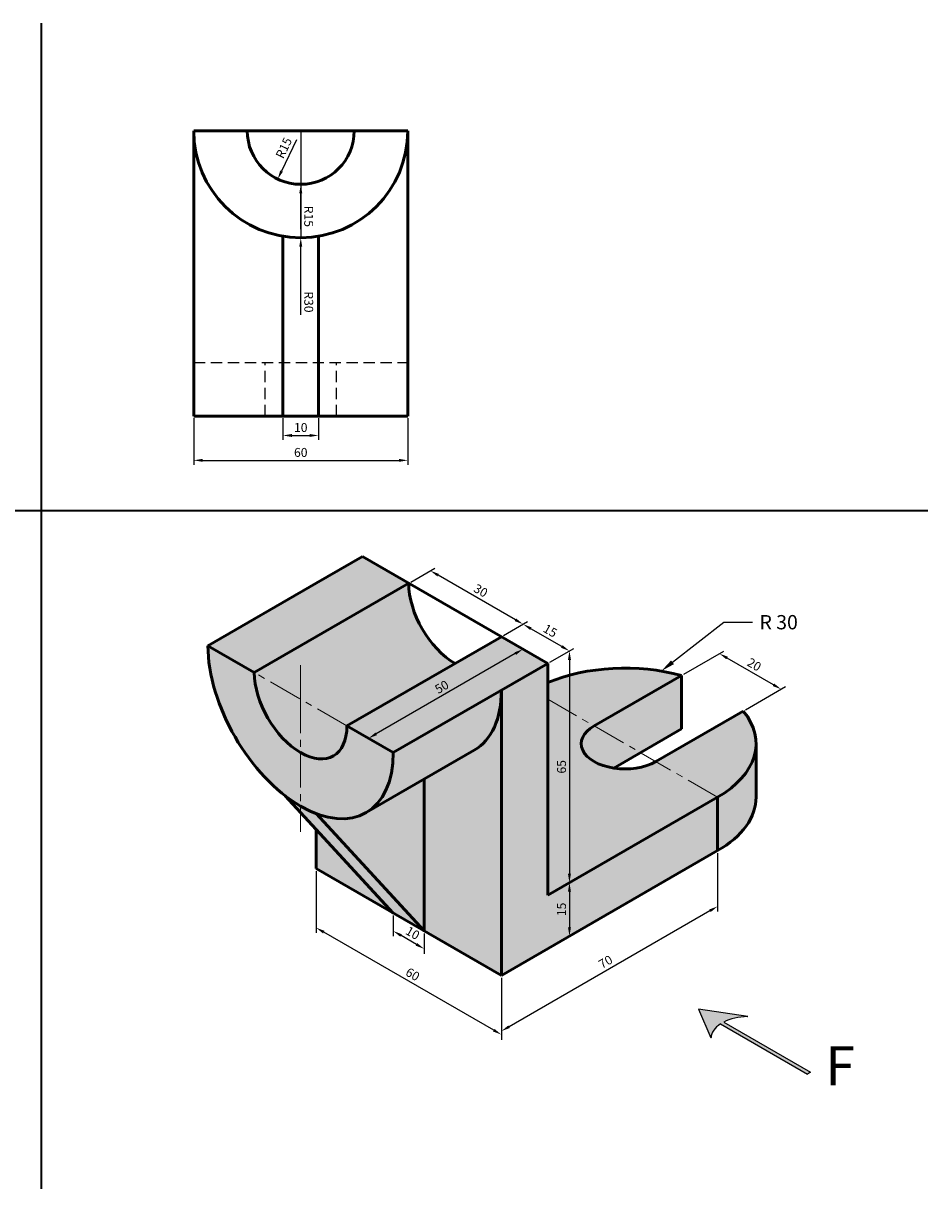
# Model space of a CAD drawing. Units: millimetres. Extents: x 2100 to 2598, y 2059 to 2386.
# Tile 1 of 1: x 2345 to 2598.5, y 2059.2 to 2386.1. Entities that reach past the tile are written whole.
import ezdxf
from ezdxf import colors
from ezdxf.entities.mleader import LeaderData, LeaderLine
from ezdxf.math import Vec2, Vec3

# ---------------------------------------------------------------- set-up
doc = ezdxf.new("R2010")
doc.units = ezdxf.units.MM
doc.linetypes.add('CENTER', pattern=[50.800000000000004, 31.75, -6.349999999999999, 6.349999999999999, -6.349999999999999])
doc.linetypes.add('HIDDEN', pattern=[9.524999999999999, 6.349999999999999, -3.174999999999999])
for name, color, linetype, lineweight in [('M-CNTR', 1, 'CENTER', 18), ('M-DIMS', 2, 'Continuous', 25), ('M-HATC', 8, 'Continuous', 18), ('M-HIDN', 4, 'HIDDEN', 25), ('M-OUTL', 7, 'Continuous', 50), ('M-SYMB', 3, 'Continuous', 25), ('M-TEXT', 3, 'Continuous', 25), ('M-TTLB', 7, 'Continuous', 35)]:
    doc.layers.add(name, color=color, linetype=linetype, lineweight=lineweight)
doc.styles.get("Standard").update_dxf_attribs({"font": 'arial.ttf'})
doc.dimstyles.new('ISO-25', dxfattribs={"dimtxt": 2.5, "dimasz": 2.5, "dimexe": 1.25, "dimexo": 0.625, "dimtad": 1, "dimtxsty": 'Standard', "dimcen": 2.5, "dimadec": 0, "dimazin": 0, "dimtfac": 1, "dimtmove": 0, "dimatfit": 3, "dimfxl": 1, "dimarcsym": 0})

# ---------------------------------------------------------------- blocks, each defined once
blk = doc.blocks.new('*D1')
at = {"layer": 'Defpoints', "color": 0, "transparency": 16777216}
for p in [(2539.605304126091, 2154.015574950749), (2478.98352586118, 2119.015574950749), (2478.98352586118, 2103.385647397557)]:
    blk.add_point(p, dxfattribs=at)
at = {"layer": 'M-DIMS', "color": 0, "lineweight": -2, "transparency": 16777216}
for p, q in [((2539.605304126091, 2153.293887114262), (2539.605304126091, 2136.942271724583)), ((2537.44024061663, 2137.135647397557), (2481.148589370641, 2104.635647397557)), ((2478.98352586118, 2118.293887114262), (2478.98352586118, 2101.942271724583))]:
    blk.add_line(p, q, dxfattribs=at)
at = {"layer": 'M-DIMS', "color": 0, "transparency": 16777216}
for points in [[(2537.231907283296, 2137.4964913158), (2537.648573949963, 2136.774803479313), (2539.605304126091, 2138.385647397557)], [(2480.940256037307, 2104.9964913158), (2481.356922703974, 2104.274803479313), (2478.98352586118, 2103.385647397557)]]:
    blk.add_solid(points, dxfattribs=at)
at = {"layer": 'M-DIMS', "color": 0, "transparency": 16777216, "insert": (2508.343698758983, 2122.532336219554), "char_height": 2.5, "attachment_point": 5, "rotation": 30.000000000000068}
blk.add_mtext('70', dxfattribs=at)
blk = doc.blocks.new('*D2')
at = {"layer": 'Defpoints', "color": 0, "transparency": 16777216}
for p in [(2427.022001634114, 2149.01557495075), (2427.022001634114, 2132.403009386933), (2478.98352586118, 2119.015574950749)]:
    blk.add_point(p, dxfattribs=at)
at = {"layer": 'M-DIMS', "color": 0, "lineweight": -2, "transparency": 16777216}
for p, q in [((2427.022001634114, 2148.293887114263), (2427.022001634114, 2130.959633713958)), ((2476.818462351719, 2103.653009386933), (2429.187065143575, 2131.153009386932)), ((2478.98352586118, 2118.293887114262), (2478.98352586118, 2100.959633713959))]:
    blk.add_line(p, q, dxfattribs=at)
at = {"layer": 'M-DIMS', "color": 0, "transparency": 16777216}
for points in [[(2429.395398476908, 2131.513853305176), (2428.978731810242, 2130.79216546869), (2427.022001634114, 2132.403009386933)], [(2477.026795685052, 2104.013853305176), (2476.610129018386, 2103.29216546869), (2478.98352586118, 2102.403009386933)]]:
    blk.add_solid(points, dxfattribs=at)
at = {"layer": 'M-DIMS', "color": 0, "transparency": 16777216, "insert": (2453.953479982299, 2119.049698208931), "char_height": 2.5, "attachment_point": 5, "rotation": 330.0000000000001}
blk.add_mtext('60', dxfattribs=at)
blk = doc.blocks.new('*D3')
at = {"layer": 'Defpoints', "color": 0, "transparency": 16777216}
for p in [(2448.672636728725, 2136.515574950749), (2448.672636728725, 2131.469743862794), (2457.332890766569, 2131.515574950749)]:
    blk.add_point(p, dxfattribs=at)
at = {"layer": 'M-DIMS', "color": 0, "lineweight": -2, "transparency": 16777216}
for p, q in [((2448.672636728725, 2135.793887114262), (2448.672636728725, 2130.026368189821)), ((2455.167827257108, 2127.719743862795), (2450.837700238186, 2130.219743862795)), ((2457.332890766569, 2130.793887114263), (2457.332890766569, 2125.026368189821))]:
    blk.add_line(p, q, dxfattribs=at)
at = {"layer": 'M-DIMS', "color": 0, "transparency": 16777216}
for points in [[(2451.046033571519, 2130.580587781038), (2450.629366904853, 2129.858899944551), (2448.672636728725, 2131.469743862794)], [(2455.376160590442, 2128.080587781038), (2454.959493923775, 2127.358899944551), (2457.332890766569, 2126.469743862795)]]:
    blk.add_solid(points, dxfattribs=at)
at = {"layer": 'M-DIMS', "color": 0, "transparency": 16777216, "insert": (2453.953479982299, 2130.616432684793), "char_height": 2.5, "attachment_point": 5, "rotation": 330.0000000000001}
blk.add_mtext('10', dxfattribs=at)
blk = doc.blocks.new('*D4')
at = {"layer": 'Defpoints', "color": 0, "transparency": 16777216}
for p in [(2491.973906917947, 2206.515574950749), (2441.723938290984, 2185.527407864297), (2448.672636728725, 2181.515574950749)]:
    blk.add_point(p, dxfattribs=at)
at = {"layer": 'M-DIMS', "color": 0, "lineweight": -2, "transparency": 16777216}
for p, q in [((2491.348906917947, 2206.876418868993), (2483.775208480207, 2211.249095700784)), ((2482.860144970745, 2209.277407864297), (2443.889001800445, 2186.777407864297)), ((2448.047636728726, 2181.876418868993), (2440.473938290984, 2186.249095700784))]:
    blk.add_line(p, q, dxfattribs=at)
at = {"layer": 'M-DIMS', "color": 0, "transparency": 16777216}
for points in [[(2482.651811637412, 2209.638251782541), (2483.068478304079, 2208.916563946054), (2485.025208480207, 2210.527407864297)], [(2443.680668467112, 2187.138251782541), (2444.097335133779, 2186.416563946053), (2441.723938290984, 2185.527407864297)]]:
    blk.add_solid(points, dxfattribs=at)
at = {"layer": 'M-DIMS', "color": 0, "transparency": 16777216, "insert": (2462.423857150943, 2199.674096686295), "char_height": 2.5, "attachment_point": 5, "rotation": 29.999999999999872}
blk.add_mtext('50', dxfattribs=at)
blk = doc.blocks.new('*D5')
at = {"layer": 'Defpoints', "color": 0, "transparency": 16777216}
for p in [(2485.074026823124, 2217.531927320627), (2478.98352586118, 2214.015574950749), (2491.973906917947, 2206.515574950749)]:
    blk.add_point(p, dxfattribs=at)
at = {"layer": 'M-DIMS', "color": 0, "lineweight": -2, "transparency": 16777216}
for p, q in [((2479.608525861181, 2214.376418868993), (2486.324026823124, 2218.253615157115)), ((2495.89934437043, 2211.281927320627), (2487.239090332585, 2216.281927320627)), ((2492.598906917947, 2206.876418868993), (2499.314407879891, 2210.753615157114))]:
    blk.add_line(p, q, dxfattribs=at)
at = {"layer": 'M-DIMS', "color": 0, "transparency": 16777216}
for points in [[(2487.447423665918, 2216.642771238871), (2487.030756999252, 2215.921083402384), (2485.074026823124, 2217.531927320627)], [(2496.107677703763, 2211.642771238871), (2495.691011037096, 2210.921083402384), (2498.064407879891, 2210.031927320627)]]:
    blk.add_solid(points, dxfattribs=at)
at = {"layer": 'M-DIMS', "color": 0, "transparency": 16777216, "insert": (2492.519933586159, 2215.428616142625), "char_height": 2.5, "attachment_point": 5, "rotation": 330.0000000000001}
blk.add_mtext('15', dxfattribs=at)
blk = doc.blocks.new('*D6')
at = {"layer": 'Defpoints', "color": 0, "transparency": 16777216}
for p in [(2491.973906917948, 2206.515574950751), (2498.064407879893, 2145.031927320629), (2491.973906917948, 2141.51557495075)]:
    blk.add_point(p, dxfattribs=at)
at = {"layer": 'M-DIMS', "color": 0, "lineweight": -2, "transparency": 16777216}
for p, q in [((2492.598906917948, 2206.876418868994), (2499.314407879893, 2210.753615157116)), ((2498.064407879893, 2207.531927320629), (2498.064407879893, 2147.531927320629)), ((2492.598906917948, 2141.876418868994), (2499.314407879893, 2145.753615157116))]:
    blk.add_line(p, q, dxfattribs=at)
at = {"layer": 'M-DIMS', "color": 0, "transparency": 16777216}
for points in [[(2497.647741213226, 2207.531927320629), (2498.481074546559, 2207.531927320629), (2498.064407879893, 2210.031927320629)], [(2497.647741213226, 2147.531927320629), (2498.481074546559, 2147.531927320629), (2498.064407879893, 2145.031927320629)]]:
    blk.add_solid(points, dxfattribs=at)
at = {"layer": 'M-DIMS', "color": 0, "transparency": 16777216, "insert": (2496.162975410588, 2177.531927320628), "char_height": 2.5, "attachment_point": 5, "rotation": 90}
blk.add_mtext('65', dxfattribs=at)
blk = doc.blocks.new('*D7')
at = {"layer": 'Defpoints', "color": 0, "transparency": 16777216}
for p in [(2459.093264709591, 2232.531927320627), (2453.002763747647, 2229.01557495075), (2478.98352586118, 2214.015574950749)]:
    blk.add_point(p, dxfattribs=at)
at = {"layer": 'M-DIMS', "color": 0, "lineweight": -2, "transparency": 16777216}
for p, q in [((2453.627763747647, 2229.376418868993), (2460.343264709591, 2233.253615157114)), ((2482.908963313662, 2218.781927320627), (2461.258328219052, 2231.281927320627)), ((2479.608525861181, 2214.376418868993), (2486.324026823123, 2218.253615157115))]:
    blk.add_line(p, q, dxfattribs=at)
at = {"layer": 'M-DIMS', "color": 0, "transparency": 16777216}
for points in [[(2461.466661552385, 2231.642771238871), (2461.049994885719, 2230.921083402384), (2459.093264709591, 2232.531927320627)], [(2483.117296646996, 2219.142771238871), (2482.70062998033, 2218.421083402384), (2485.074026823124, 2217.531927320627)]]:
    blk.add_solid(points, dxfattribs=at)
at = {"layer": 'M-DIMS', "color": 0, "transparency": 16777216, "insert": (2473.03478833116, 2226.679354568106), "char_height": 2.5, "attachment_point": 5, "rotation": 330.0000000000001}
blk.add_mtext('30', dxfattribs=at)
blk = doc.blocks.new('*D8')
at = {"layer": 'Defpoints', "color": 0, "transparency": 16777216}
for p in [(2540.093305136287, 2209.297322465351), (2529.459185402545, 2203.157710574481), (2546.779693478234, 2193.15771057448)]:
    blk.add_point(p, dxfattribs=at)
at = {"layer": 'M-DIMS', "color": 0, "lineweight": -2, "transparency": 16777216}
for p, q in [((2530.084185402545, 2203.518554492724), (2541.343305136287, 2210.019010301838)), ((2555.248749702514, 2200.547322465352), (2542.258368645748, 2208.047322465351)), ((2547.404693478234, 2193.518554492724), (2558.663813211976, 2200.019010301839))]:
    blk.add_line(p, q, dxfattribs=at)
at = {"layer": 'M-DIMS', "color": 0, "transparency": 16777216}
for points in [[(2542.466701979082, 2208.408166383595), (2542.050035312414, 2207.686478547108), (2540.093305136287, 2209.297322465351)], [(2555.457083035848, 2200.908166383595), (2555.040416369181, 2200.186478547108), (2557.413813211976, 2199.297322465351)]]:
    blk.add_solid(points, dxfattribs=at)
at = {"layer": 'M-DIMS', "color": 0, "transparency": 16777216, "insert": (2549.704275408783, 2205.94401128735), "char_height": 2.5, "attachment_point": 5, "rotation": 330.0000000000001}
blk.add_mtext('20', dxfattribs=at)
blk = doc.blocks.new('*D9')
at = {"layer": 'Defpoints', "color": 0, "transparency": 16777216}
for p in [(2491.973906917948, 2141.51557495075), (2498.064407879894, 2130.031927320629), (2491.973906917948, 2126.515574950751)]:
    blk.add_point(p, dxfattribs=at)
at = {"layer": 'M-DIMS', "color": 0, "lineweight": -2, "transparency": 16777216}
for p, q in [((2492.598906917948, 2141.876418868994), (2499.314407879894, 2145.753615157116)), ((2498.064407879894, 2142.531927320629), (2498.064407879894, 2132.53192732063)), ((2492.598906917948, 2126.876418868994), (2499.314407879894, 2130.753615157117))]:
    blk.add_line(p, q, dxfattribs=at)
at = {"layer": 'M-DIMS', "color": 0, "transparency": 16777216}
for points in [[(2497.647741213227, 2142.531927320629), (2498.48107454656, 2142.531927320629), (2498.064407879894, 2145.031927320629)], [(2497.647741213227, 2132.53192732063), (2498.48107454656, 2132.53192732063), (2498.064407879894, 2130.031927320629)]]:
    blk.add_solid(points, dxfattribs=at)
at = {"layer": 'M-DIMS', "color": 0, "transparency": 16777216, "insert": (2496.16297541059, 2137.531927320629), "char_height": 2.5, "attachment_point": 5, "rotation": 90}
blk.add_mtext('15', dxfattribs=at)
blk = doc.blocks.new('*D15')
at = {"layer": 'Defpoints', "color": 0, "transparency": 16777216}
for p in [(2417.737806239899, 2275.948119333525), (2427.737806239898, 2275.948119333525), (2427.737806239898, 2270.485342262566)]:
    blk.add_point(p, dxfattribs=at)
at = {"layer": 'M-DIMS', "color": 0, "lineweight": -2, "transparency": 16777216}
for p, q in [((2417.737806239899, 2275.323119333525), (2417.737806239899, 2269.235342262566)), ((2427.737806239898, 2275.323119333525), (2427.737806239898, 2269.235342262566)), ((2420.237806239899, 2270.485342262566), (2425.237806239899, 2270.485342262566))]:
    blk.add_line(p, q, dxfattribs=at)
at = {"layer": 'M-DIMS', "color": 0, "transparency": 16777216}
for points in [[(2420.237806239899, 2270.902008929232), (2420.237806239899, 2270.068675595899), (2417.737806239899, 2270.485342262566)], [(2425.237806239899, 2270.902008929232), (2425.237806239899, 2270.068675595899), (2427.737806239898, 2270.485342262566)]]:
    blk.add_solid(points, dxfattribs=at)
at = {"layer": 'M-DIMS', "color": 0, "transparency": 16777216, "insert": (2422.737806239898, 2272.38677473187), "char_height": 2.5, "attachment_point": 5}
blk.add_mtext('10', dxfattribs=at)
blk = doc.blocks.new('*D16')
at = {"layer": 'Defpoints', "color": 0, "transparency": 16777216}
for p in [(2392.737806239899, 2275.948119333525), (2452.737806239899, 2275.948119333525), (2452.737806239899, 2263.507971917901)]:
    blk.add_point(p, dxfattribs=at)
at = {"layer": 'M-DIMS', "color": 0, "lineweight": -2, "transparency": 16777216}
for p, q in [((2392.737806239899, 2275.323119333525), (2392.737806239899, 2262.257971917901)), ((2452.737806239899, 2275.323119333525), (2452.737806239899, 2262.257971917901)), ((2395.237806239899, 2263.507971917901), (2450.237806239899, 2263.507971917901))]:
    blk.add_line(p, q, dxfattribs=at)
at = {"layer": 'M-DIMS', "color": 0, "transparency": 16777216}
for points in [[(2395.237806239899, 2263.924638584568), (2395.237806239899, 2263.091305251235), (2392.737806239899, 2263.507971917901)], [(2450.237806239899, 2263.924638584568), (2450.237806239899, 2263.091305251235), (2452.737806239899, 2263.507971917901)]]:
    blk.add_solid(points, dxfattribs=at)
at = {"layer": 'M-DIMS', "color": 0, "transparency": 16777216, "insert": (2422.737806239898, 2265.409404387206), "char_height": 2.5, "attachment_point": 5}
blk.add_mtext('60', dxfattribs=at)
blk = doc.blocks.new('*D17')
at = {"layer": 'Defpoints', "color": 0, "transparency": 16777216}
for p in [(2422.737806239896, 2355.948119333517), (2416.274107555597, 2342.412218945352)]:
    blk.add_point(p, dxfattribs=at)
at = {"layer": 'M-DIMS', "color": 0, "lineweight": -2, "transparency": 16777216}
blk.add_line((2421.549561495412, 2353.459766567759), (2417.351390669647, 2344.668202343381), dxfattribs=at)
at = {"layer": 'M-DIMS', "color": 0, "transparency": 16777216}
blk.add_solid([(2416.975393436643, 2344.847749529055), (2417.727387902653, 2344.488655157705), (2416.274107555597, 2342.412218945352)], dxfattribs=at)
at = {"layer": 'M-DIMS', "color": 0, "transparency": 16777216, "insert": (2418.273277606266, 2351.01132859126), "char_height": 2.5, "attachment_point": 5, "rotation": 64.47446902836414}
blk.add_mtext('R15', dxfattribs=at)
blk = doc.blocks.new('*D22')
at = {"layer": 'Defpoints', "color": 0, "transparency": 16777216}
for p in [(2422.737806000001, 2355.948119000002), (2422.738000000001, 2340.948119000001)]:
    blk.add_point(p, dxfattribs=at)
at = {"layer": 'M-DIMS', "color": 0, "lineweight": -2, "transparency": 16777216}
for p, q in [((2422.737806000001, 2355.948119000002), (2422.738000000001, 2340.948119000001)), ((2422.738163234812, 2328.326870706377), (2422.738032333334, 2338.44811900021))]:
    blk.add_line(p, q, dxfattribs=at)
at = {"layer": 'M-DIMS', "color": 0, "transparency": 16777216}
blk.add_solid([(2423.154698999966, 2338.448124389099), (2422.321365666702, 2338.448113611321), (2422.738000000001, 2340.948119000001)], dxfattribs=at)
at = {"layer": 'M-DIMS', "color": 0, "transparency": 16777216, "insert": (2424.639548869146, 2331.948143592613), "char_height": 2.5, "attachment_point": 5, "rotation": 270.00074102541396}
blk.add_mtext('R15', dxfattribs=at)
blk = doc.blocks.new('*D23')
at = {"layer": 'Defpoints', "color": 0, "transparency": 16777216}
for p in [(2422.737806000003, 2355.948119000001), (2422.738000000002, 2325.948119000003)]:
    blk.add_point(p, dxfattribs=at)
at = {"layer": 'M-DIMS', "color": 0, "lineweight": -2, "transparency": 16777216}
for p, q in [((2422.737806000003, 2355.948119000001), (2422.738000000002, 2325.948119000003)), ((2422.738139729186, 2304.340513270576), (2422.73801616667, 2323.448119000055))]:
    blk.add_line(p, q, dxfattribs=at)
at = {"layer": 'M-DIMS', "color": 0, "transparency": 16777216}
blk.add_solid([(2423.154682833327, 2323.448121694499), (2422.321349500011, 2323.44811630561), (2422.738000000002, 2325.948119000003)], dxfattribs=at)
at = {"layer": 'M-DIMS', "color": 0, "transparency": 16777216, "insert": (2424.640401529567, 2307.948131301821), "char_height": 2.5, "attachment_point": 5, "rotation": 270.00037051270704}
blk.add_mtext('R30', dxfattribs=at)

msp = doc.modelspace()

# ---------------------------------------------------------------- hatches: boundary and pattern name
at = {"layer": 'M-HATC'}
h = msp.add_hatch(color=256, dxfattribs=at)
h.dxf.hatch_style = 1
edge = h.paths.add_edge_path()
edge.add_ellipse((2453.002763747647, 2214.015574950749), major_axis=(18.37117307087393, -31.81980515339472), ratio=0.5773502691896212, start_angle=360, end_angle=390)
edge.add_line((2478.98352586118, 2199.015574950749), (2448.672636728725, 2181.515574950749))
edge.add_ellipse((2422.691874615191, 2196.515574950749), major_axis=(18.37117307087387, -31.81980515339462), ratio=0.5773502691896232, start_angle=359.9999999999999, end_angle=390, ccw=False)
edge.add_line((2441.063047686065, 2164.695769797355), (2471.373936818521, 2182.195769797355))
h.paths.add_polyline_path([(2478.98352586118, 2199.015574950749), (2491.973906917948, 2206.515574950749), (2478.98352586118, 2214.01557495075), (2435.682255671958, 2189.01557495075), (2448.672636728725, 2181.515574950749)])
edge = h.paths.add_edge_path()
edge.add_ellipse((2453.002763747647, 2214.015574950749), major_axis=(18.37117307087393, -31.81980515339472), ratio=0.5773502691896212, start_angle=360, end_angle=390, ccw=False)
edge.add_line((2471.373936818521, 2182.195769797355), (2457.332890766569, 2174.089168079557))
edge.add_line((2457.332890766569, 2174.089168079557), (2457.332890766569, 2131.515574950749))
edge.add_line((2457.332890766569, 2131.515574950749), (2478.98352586118, 2119.015574950749))
edge.add_line((2478.98352586118, 2119.015574950749), (2478.98352586118, 2199.015574950749))
h.paths.add_polyline_path([(2491.973906917947, 2206.515574950749), (2478.98352586118, 2199.015574950749), (2478.98352586118, 2119.015574950749), (2539.605304126091, 2154.015574950749), (2539.605304126091, 2169.01557495075), (2491.973906917947, 2141.51557495075)])
h.paths.add_polyline_path([(2539.605304126091, 2169.01557495075), (2491.973906917947, 2196.51557495075), (2491.973906917947, 2141.51557495075)], flags=17)
edge = h.paths.add_edge_path()
edge.add_ellipse((2513.624542012558, 2184.01557495075), major_axis=(-36.74234614174767, 0), ratio=0.5773502691896243, start_angle=510, end_angle=540)
edge.add_ellipse((2513.624542012558, 2184.01557495075), major_axis=(-36.74234614174767, 0), ratio=0.5773502691896243, start_angle=540, end_angle=195.4155559431911)
edge.add_line((2546.779693478235, 2193.157710574481), (2522.284796050402, 2179.015574950749))
edge.add_line((2522.284796050402, 2179.015574950749), (2539.605304126091, 2169.01557495075))
edge = h.paths.add_edge_path(flags=17)
edge.add_ellipse((2513.624542012558, 2184.01557495075), major_axis=(-36.74234614174767, 0), ratio=0.5773502691896243, start_angle=230.4019697012312, end_angle=321.6340594852775)
edge.add_line((2491.973906917947, 2201.154711451752), (2491.973906917947, 2196.51557495075))
edge.add_line((2491.973906917947, 2196.51557495075), (2504.964287974714, 2189.01557495075))
edge.add_line((2504.964287974714, 2189.01557495075), (2529.459185402545, 2203.15771057448))
edge = h.paths.add_edge_path(flags=16)
edge.add_line((2517.95466903148, 2181.515574950749), (2504.964287974714, 2189.01557495075))
edge.add_ellipse((2513.624542012558, 2184.01557495075), major_axis=(-12.24744871391589, 0), ratio=0.5773502691896119, start_angle=329.9999999999987, end_angle=425.1039093610203)
edge.add_line((2510.45466903148, 2177.185447931827), (2517.95466903148, 2181.515574950749))
edge = h.paths.add_edge_path(flags=16)
edge.add_ellipse((2513.624542012558, 2184.01557495075), major_axis=(-12.24744871391589, 0), ratio=0.5773502691896119, start_angle=425.1039093610203, end_angle=510.0000000000001)
edge.add_line((2522.284796050402, 2179.015574950749), (2517.95466903148, 2181.515574950749))
edge.add_line((2517.95466903148, 2181.515574950749), (2510.45466903148, 2177.185447931827))
edge = h.paths.add_edge_path()
edge.add_line((2550.366888154305, 2169.01557495075), (2550.366888154305, 2184.01557495075))
edge.add_ellipse((2513.624542012558, 2184.01557495075), major_axis=(-36.74234614174767, 0), ratio=0.5773502691896243, start_angle=510.0000000000001, end_angle=540, ccw=False)
edge.add_line((2539.605304126091, 2169.01557495075), (2539.605304126091, 2154.015574950749))
edge.add_ellipse((2513.624542012558, 2169.01557495075), major_axis=(-36.74234614174767, 0), ratio=0.5773502691896243, start_angle=510, end_angle=540)
h.paths.add_polyline_path([(2478.98352586118, 2119.015574950749), (2478.98352586118, 2199.015574950749), (2448.672636728725, 2181.515574950749), (2435.682255671958, 2189.01557495075), (2422.691874615191, 2196.515574950749), (2422.691874615191, 2164.732375880323), (2448.672636728725, 2136.515574950749)], flags=17)
edge = h.paths.add_edge_path()
edge.add_ellipse((2422.691874615191, 2196.515574950749), major_axis=(9.185586535436936, -15.90990257669731), ratio=0.5773502691896232, start_angle=210.0000000000001, end_angle=329.99999999999994, ccw=False)
edge.add_line((2409.701493558425, 2204.01557495075), (2396.711112501658, 2211.51557495075))
edge.add_ellipse((2422.691874615191, 2196.515574950749), major_axis=(18.37117307087387, -31.81980515339462), ratio=0.5773502691896232, start_angle=210, end_angle=320.9153690765151)
edge.add_ellipse((2422.691874615191, 2196.515574950749), major_axis=(18.37117307087387, -31.81980515339462), ratio=0.5773502691896232, start_angle=320.9153690765151, end_angle=329.9999999999999)
edge.add_line((2422.691874615191, 2166.51557495075), (2422.691874615191, 2181.515574950749))
h.paths.add_polyline_path([(2453.002763747647, 2229.01557495075), (2440.012382690881, 2236.515574950749), (2427.022001634114, 2229.01557495075), (2396.711112501658, 2211.51557495075), (2409.701493558425, 2204.01557495075)])
edge = h.paths.add_edge_path()
edge.add_ellipse((2422.691874615191, 2196.515574950749), major_axis=(9.185586535436936, -15.90990257669731), ratio=0.5773502691896232, start_angle=329.9999999999999, end_angle=390)
edge.add_line((2435.682255671958, 2189.01557495075), (2422.691874615191, 2196.515574950749))
edge.add_line((2422.691874615191, 2196.515574950749), (2422.691874615191, 2181.515574950749))
h.paths.add_polyline_path([(2478.98352586118, 2199.015574950749), (2448.672636728725, 2181.515574950749), (2435.682255671958, 2189.01557495075), (2422.691874615191, 2196.515574950749), (2422.691874615191, 2181.515574950749), (2422.691874615191, 2166.51557495075), (2422.691874615191, 2164.732375880323), (2448.672636728725, 2136.515574950749), (2478.98352586118, 2119.015574950749)], flags=17)
h.paths.add_polyline_path([(2427.022001634114, 2160.029575725394), (2427.022001634114, 2149.01557495075), (2448.672636728725, 2136.515574950749)], flags=0)
h = msp.add_hatch(color=256, dxfattribs=at)
h.dxf.hatch_style = 1
edge = h.paths.add_edge_path()
edge.add_ellipse((2465.993144804414, 2221.51557495075), major_axis=(9.185586535436936, -15.90990257669731), ratio=0.5773502691896232, start_angle=210.0000000000001, end_angle=329.99999999999994, ccw=False)
edge.add_line((2453.002763747647, 2229.01557495075), (2409.701493558425, 2204.01557495075))
edge.add_line((2409.701493558425, 2204.01557495075), (2435.682255671958, 2189.01557495075))
edge.add_line((2435.682255671958, 2189.01557495075), (2465.993144804413, 2206.515574950749))
edge = h.paths.add_edge_path()
edge.add_line((2422.691874615191, 2196.515574950749), (2409.701493558425, 2204.01557495075))
edge.add_ellipse((2422.691874615191, 2196.515574950749), major_axis=(9.185586535436936, -15.90990257669731), ratio=0.5773502691896232, start_angle=210, end_angle=329.9999999999999)
edge.add_line((2422.691874615191, 2181.515574950749), (2422.691874615191, 2196.515574950749))
edge = h.paths.add_edge_path()
edge.add_ellipse((2422.691874615191, 2196.515574950749), major_axis=(9.185586535436936, -15.90990257669731), ratio=0.5773502691896232, start_angle=329.9999999999999, end_angle=390)
edge.add_line((2435.682255671958, 2189.01557495075), (2422.691874615191, 2196.515574950749))
edge.add_line((2422.691874615191, 2196.515574950749), (2422.691874615191, 2181.515574950749))
h.paths.add_polyline_path([(2529.459185402545, 2203.157710574481), (2504.964287974714, 2189.01557495075), (2517.95466903148, 2181.515574950749), (2529.459185402545, 2188.157710574481)])
edge = h.paths.add_edge_path()
edge.add_ellipse((2513.624542012558, 2184.01557495075), major_axis=(-12.24744871391589, 0), ratio=0.5773502691896119, start_angle=329.9999999999987, end_angle=425.1039093610203)
edge.add_line((2510.45466903148, 2177.185447931827), (2517.95466903148, 2181.515574950749))
edge.add_line((2517.95466903148, 2181.515574950749), (2504.964287974714, 2189.01557495075))
edge = h.paths.add_edge_path()
edge.add_line((2457.332890766569, 2174.089168079557), (2441.063047686065, 2164.695769797355))
edge.add_ellipse((2422.691874615191, 2196.515574950749), major_axis=(18.37117307087387, -31.81980515339462), ratio=0.5773502691896232, start_angle=337.68717287009406, end_angle=359.9999999999999, ccw=False)
edge.add_line((2427.022001634114, 2164.435176035252), (2457.332890766569, 2131.515574950749))
edge.add_line((2457.332890766569, 2131.515574950749), (2457.332890766569, 2174.089168079557))
edge = h.paths.add_edge_path()
edge.add_ellipse((2422.691874615191, 2196.515574950749), major_axis=(18.37117307087387, -31.81980515339462), ratio=0.5773502691896232, start_angle=329.99999999999994, end_angle=337.68717287009406, ccw=False)
edge.add_line((2422.691874615191, 2166.51557495075), (2422.691874615191, 2164.732375880323))
edge.add_line((2422.691874615191, 2164.732375880323), (2448.672636728725, 2136.515574950749))
edge.add_line((2448.672636728725, 2136.515574950749), (2457.332890766569, 2131.515574950749))
edge.add_line((2457.332890766569, 2131.515574950749), (2427.022001634114, 2164.435176035252))
edge = h.paths.add_edge_path()
edge.add_ellipse((2422.691874615191, 2196.515574950749), major_axis=(18.37117307087387, -31.81980515339462), ratio=0.5773502691896232, start_angle=320.9153690765151, end_angle=329.99999999999994, ccw=False)
edge.add_line((2418.361747596269, 2169.435176035252), (2422.691874615191, 2164.732375880323))
edge.add_line((2422.691874615191, 2164.732375880323), (2422.691874615191, 2166.51557495075))
h = msp.add_hatch(color=256, dxfattribs=at)
h.dxf.hatch_style = 1
edge = h.paths.add_edge_path()
edge.add_ellipse((2422.691874615191, 2196.515574950749), major_axis=(18.37117307087387, -31.81980515339462), ratio=0.5773502691896232, start_angle=359.9999999999999, end_angle=390)
edge.add_line((2448.672636728725, 2181.515574950749), (2435.682255671958, 2189.01557495075))
edge.add_ellipse((2422.691874615191, 2196.515574950749), major_axis=(9.185586535436936, -15.90990257669731), ratio=0.5773502691896232, start_angle=329.99999999999994, end_angle=390, ccw=False)
edge.add_line((2422.691874615191, 2181.515574950749), (2422.691874615191, 2166.51557495075))
edge.add_ellipse((2422.691874615191, 2196.515574950749), major_axis=(18.37117307087387, -31.81980515339462), ratio=0.5773502691896232, start_angle=329.9999999999999, end_angle=337.6871728700941)
edge.add_ellipse((2422.691874615191, 2196.515574950749), major_axis=(18.37117307087387, -31.81980515339462), ratio=0.5773502691896232, start_angle=337.6871728700941, end_angle=359.9999999999999)
h.paths.add_polyline_path([(2427.022001634114, 2160.029575725394), (2427.022001634114, 2149.01557495075), (2448.672636728725, 2136.515574950749)])
at = {"layer": 'M-SYMB'}
h = msp.add_hatch(color=256, dxfattribs=at)
h.dxf.hatch_style = 1
edge = h.paths.add_edge_path()
edge.add_ellipse((2548.340327794889, 2101.348676846816), major_axis=(-10.59557621008401, 0), ratio=0.5773502691896403, start_angle=273.4886162533513, end_angle=327.04442488872957, ccw=False)
edge.add_line((2547.967624843714, 2107.46224993555), (2548.055619139272, 2107.513053465777))
edge.add_line((2548.055619139272, 2107.513053465777), (2534.199212678721, 2109.513053465777))
edge.add_line((2534.199212678721, 2109.513053465777), (2537.663314293859, 2101.513053465778))
edge.add_line((2537.663314293859, 2101.513053465778), (2537.751308589416, 2101.563856996005))
edge.add_ellipse((2548.340327794889, 2101.348676846816), major_axis=(-10.59557621008401, 0), ratio=0.5773502691896403, start_angle=332.78955523151785, end_angle=358.8358489575538, ccw=False)
edge.add_line((2540.427634778182, 2105.417072290027), (2564.810455235822, 2091.339644335207))
edge.add_line((2564.810455235822, 2091.339644335207), (2565.676480639606, 2091.839644335206))
edge.add_line((2565.676480639606, 2091.839644335206), (2541.293660181966, 2105.917072290028))

# ---------------------------------------------------------------- linework, layer by layer
at = {"layer": 'M-CNTR', "ltscale": 0.3}
for p, q in [((2422.691874615191, 2196.515574950749), (2422.691874615191, 2206.954988744756)), ((2435.682255671958, 2189.01557495075), (2409.701493558425, 2204.01557495075)), ((2422.691874615191, 2196.515574950749), (2422.691874615191, 2159.288783772107)), ((2539.605304126091, 2169.01557495075), (2491.973906917947, 2196.51557495075))]:
    msp.add_line(p, q, dxfattribs=at)
at = {"layer": 'M-HIDN', "ltscale": 0.5}
for p, q in [((2392.737806239899, 2290.948119333525), (2452.737806239899, 2290.948119333525)), ((2412.737806239899, 2275.948119333525), (2412.737806239899, 2290.948119333526)), ((2432.737806239899, 2275.948119333525), (2432.737806239899, 2290.948119333526))]:
    msp.add_line(p, q, dxfattribs=at)
at = {"layer": 'M-OUTL'}
for p, q in [((2452.737806239899, 2355.948119333525), (2392.737806239899, 2355.948119333525)), ((2392.737806239899, 2355.948119333525), (2392.737806239899, 2275.948119333525)), ((2452.737806239899, 2275.948119333525), (2452.737806239899, 2355.948119333525)), ((2417.737806239899, 2275.948119333525), (2417.737806239899, 2326.367720418027)), ((2427.737806239898, 2275.948119333525), (2427.737806239898, 2326.367720418027)), ((2392.737806239899, 2275.948119333525), (2452.737806239899, 2275.948119333525)), ((2440.012382690881, 2236.515574950749), (2427.022001634114, 2229.01557495075)), ((2491.973906917947, 2206.515574950749), (2440.012382690881, 2236.515574950749)), ((2396.711112501658, 2211.51557495075), (2427.022001634114, 2229.01557495075)), ((2409.701493558425, 2204.01557495075), (2453.002763747647, 2229.01557495075)), ((2435.682255671958, 2189.01557495075), (2478.98352586118, 2214.01557495075)), ((2409.701493558425, 2204.01557495075), (2396.711112501658, 2211.51557495075)), ((2491.973906917948, 2206.515574950749), (2448.672636728725, 2181.515574950749)), ((2478.98352586118, 2199.015574950749), (2491.973906917947, 2206.515574950749)), ((2491.973906917947, 2206.515574950749), (2491.973906917947, 2141.51557495075)), ((2504.964287974714, 2189.01557495075), (2529.459185402545, 2203.157710574481)), ((2529.459185402545, 2203.15771057448), (2529.459185402545, 2188.157710574481)), ((2478.98352586118, 2119.015574950749), (2478.98352586118, 2199.015574950749)), ((2522.284796050402, 2179.015574950749), (2546.779693478234, 2193.15771057448)), ((2448.672636728725, 2181.515574950749), (2435.682255671958, 2189.01557495075)), ((2510.45466903148, 2177.185447931827), (2529.459185402545, 2188.157710574481)), ((2550.366888154305, 2184.01557495075), (2550.366888154305, 2169.01557495075)), ((2441.063047686065, 2164.695769797355), (2471.373936818521, 2182.195769797355)), ((2457.332890766569, 2131.515574950749), (2457.332890766569, 2174.089168079557)), ((2418.361747596269, 2169.435176035252), (2448.672636728725, 2136.515574950749)), ((2491.973906917947, 2141.51557495075), (2539.605304126091, 2169.01557495075)), ((2539.605304126091, 2154.015574950749), (2539.605304126091, 2169.01557495075)), ((2427.022001634114, 2164.435176035252), (2457.332890766569, 2131.515574950749)), ((2427.022001634114, 2149.01557495075), (2427.022001634114, 2160.029575725394)), ((2478.98352586118, 2119.015574950749), (2539.605304126091, 2154.015574950749)), ((2478.98352586118, 2119.015574950749), (2427.022001634114, 2149.01557495075))]:
    msp.add_line(p, q, dxfattribs=at)
for radius in [30, 15]:
    msp.add_arc((2422.737806239898, 2355.948119333525), radius, 180, 0, dxfattribs=at)
for centre, major_axis, ratio, start_param, end_param in [((2465.993144804414, 2221.51557495075), (9.185586535436935, -15.90990257669731), 0.5773502691896232, 3.926990816987244, 5.497787143782134), ((2422.691874615191, 2196.515574950749), (18.37117307087387, -31.81980515339462), 0.5773502691896232, 3.926990816987244, 7.068583470577037), ((2422.691874615191, 2196.515574950749), (9.185586535436935, -15.90990257669731), 0.5773502691896232, 3.926990816987244, 7.068583470577037), ((2513.624542012558, 2184.01557495075), (-36.74234614174767, 0), 0.5773502691896243, 10.55001303362094, 11.62571153362883), ((2453.002763747647, 2214.015574950749), (18.37117307087393, -31.81980515339472), 0.5773502691896212, 6.283185307179586, 7.068583470577038), ((2513.624542012558, 2184.01557495075), (-36.74234614174767, 0), 0.5773502691896243, 8.63937979737193, 9.87033921471217), ((2513.624542012558, 2184.01557495075), (-12.24744871391589, 0), 0.5773502691896119, 5.497787143782101, 8.639379797371921), ((2513.624542012558, 2169.01557495075), (-36.74234614174767, 0), 0.5773502691896243, 8.63937979737193, 9.42477796076938)]:
    msp.add_ellipse(centre, major_axis=major_axis, ratio=ratio, start_param=start_param, end_param=end_param, dxfattribs=at)
at = {"layer": 'M-SYMB'}
for p, q in [((2548.055619139272, 2107.513053465777), (2534.199212678721, 2109.513053465777)), ((2534.199212678721, 2109.513053465777), (2537.663314293859, 2101.513053465778)), ((2541.293660181966, 2105.917072290028), (2565.676480639607, 2091.839644335206)), ((2547.967624843714, 2107.46224993555), (2548.055619139272, 2107.513053465777)), ((2540.427634778182, 2105.417072290027), (2564.810455235822, 2091.339644335207)), ((2537.751308589416, 2101.563856996005), (2537.663314293859, 2101.513053465778)), ((2565.676480639606, 2091.839644335206), (2564.810455235822, 2091.339644335207))]:
    msp.add_line(p, q, dxfattribs=at)
for start_param, end_param in [(4.747571573991061, 5.439959815441913), (5.555614472122336, 6.248002713573198)]:
    msp.add_ellipse((2548.340327794889, 2101.348676846816), major_axis=(-10.59557621008401, 0), ratio=0.5773502691896403, start_param=start_param, end_param=end_param, dxfattribs=at)
at = {"layer": 'M-TTLB'}
for p, q in [((2349.945118950154, 2386.11208483271), (2349.945118950154, 2059.182228359433)), ((2100.255876839101, 2249.403035994022), (2598.481187377458, 2249.403035994022))]:
    msp.add_line(p, q, dxfattribs=at)

# ---------------------------------------------------------------- texts
at = {"layer": 'M-TEXT', "insert": (2569.80719285121, 2099.135644731203), "char_height": 11, "attachment_point": 1}
msp.add_mtext_dynamic_manual_height_columns('F', width=9.604999005729042, gutter_width=12.5, heights=[0], dxfattribs=at)

# ---------------------------------------------------------------- dimensions: what is measured, and where the dimension line sits
at = {"layer": 'M-DIMS'}
for center, mpoint, override, picture, middle in [((2422.737806239896, 2355.948119333517), (2416.274107555597, 2342.412218945352), {"dimclrd": 0, "dimclre": 0, "dimclrt": 0}, '*D17', (2419.989117639555, 2350.191976154584)), ((2422.737806000003, 2355.948119000001), (2422.738000000002, 2325.948119000003), {"dimdec": 0, "dimlfac": 1, "dimrnd": 0, "dimzin": 0, "dimdsep": 46, "dimlunit": 2}, '*D23', (2422.738116400002, 2307.948119000377)), ((2422.737806000001, 2355.948119000002), (2422.738000000001, 2340.948119000001), {"dimdec": 0, "dimlfac": 1, "dimrnd": 0, "dimzin": 0, "dimdsep": 46, "dimlunit": 2}, '*D22', (2422.738116400001, 2331.948119000753))]:
    dim = msp.add_radius_dim(center=center, mpoint=mpoint, dimstyle='ISO-25', override=override, dxfattribs=at)
    dim.commit()
    dim.dimension.update_dxf_attribs({"geometry": picture, "text_midpoint": middle, "dimtype": 164})
for p1, p2, distance, picture, middle in [((2392.737806239899, 2275.948119333525), (2452.737806239899, 2275.948119333525), -12.44014741562387, '*D16', (2422.737806239898, 2265.409404387206)), ((2417.737806239899, 2275.948119333525), (2427.737806239898, 2275.948119333525), -5.462777070958964, '*D15', (2422.737806239898, 2272.38677473187)), ((2478.98352586118, 2214.015574950749), (2453.002763747647, 2229.01557495075), -6.09050096194329, '*D7', (2473.03478833116, 2226.679354568106)), ((2491.973906917947, 2206.515574950749), (2478.98352586118, 2214.015574950749), -6.090500961943756, '*D5', (2492.519933586159, 2215.428616142625)), ((2491.973906917947, 2206.515574950749), (2448.672636728725, 2181.515574950749), -6.94869843774178, '*D4', (2462.423857150943, 2199.674096686295)), ((2491.973906917947, 2206.515574950749), (2491.973906917947, 2141.51557495075), 6.090500961946418, '*D6', (2496.162975410588, 2177.531927320628)), ((2546.779693478234, 2193.15771057448), (2529.459185402545, 2203.157710574481), -10.634119733741908, '*D8', (2549.704275408783, 2205.94401128735)), ((2539.605304126091, 2154.015574950749), (2478.98352586118, 2119.015574950749), 13.535914320374571, '*D1', (2508.343698758983, 2122.532336219554)), ((2478.98352586118, 2119.015574950749), (2427.022001634114, 2149.01557495075), 14.38690380029999, '*D2', (2453.953479982299, 2119.049698208931)), ((2491.973906917947, 2141.51557495075), (2491.973906917948, 2126.51557495075), 6.090500961946284, '*D9', (2496.16297541059, 2137.531927320629)), ((2457.332890766569, 2131.515574950749), (2448.672636728725, 2136.515574950749), 4.369817905374134, '*D3', (2453.953479982299, 2130.616432684793))]:
    dim = msp.add_aligned_dim(p1=p1, p2=p2, distance=distance, dimstyle='ISO-25', override={"dimclrd": 0, "dimclre": 0, "dimclrt": 0}, dxfattribs=at)
    dim.commit()
    dim.dimension.update_dxf_attribs({"geometry": picture, "text_midpoint": middle})

# ---------------------------------------------------------------- leaders
at = {"layer": 'M-TEXT'}
ml = msp.add_multileader_mtext('Standard', dxfattribs=at)
ml.set_content('R 30', color=256)
ml.set_leader_properties()
ml.build(insert=Vec2(0, 0))
ctx = ml.context
ctx.base_point, ctx.plane_origin = Vec3(2549.338073584137, 2218.066737735306), Vec3(2544.854974941666, 2228.593633921848)
notes = []
notes.append((ctx, [(0, (1, 1, 0), (2541.338073584137, 2218.066737735306), (1, 0), 8, [(0, [(2523.799943277873, 2204.399074888116)], 0, [])])]))
ctx.mtext.insert, ctx.mtext.width, ctx.mtext.defined_height, ctx.mtext.flow_direction = Vec3(2551.338073584137, 2220.102208403791), 22.08245904546129, 6.639661833263744, 5
for ctx, leaders in notes:
    for number, flags, end, landing, length, lines in leaders:
        leader = LeaderData()
        leader.index, (leader.has_last_leader_line, leader.has_dogleg_vector, leader.attachment_direction) = number, flags
        leader.last_leader_point, leader.dogleg_vector, leader.dogleg_length = Vec3(end), Vec3(landing), length
        for number, points, colour, breaks in lines:
            line = LeaderLine()
            line.index, line.vertices, line.color, line.breaks = number, Vec3.list(points), colors.encode_raw_color(colour), breaks
            leader.lines.append(line)
        ctx.leaders.append(leader)

doc.saveas('drawing.dxf')
